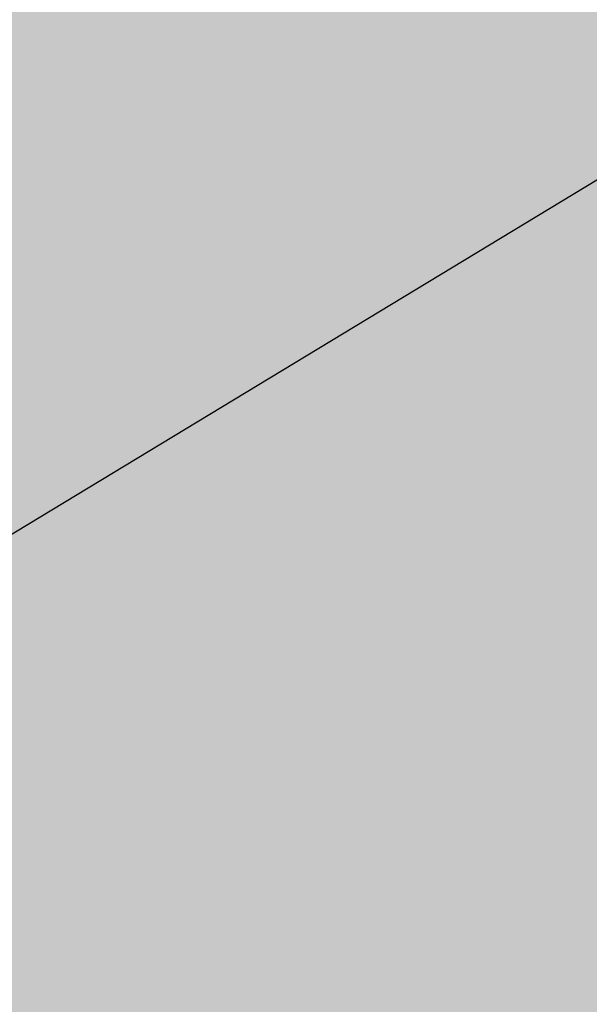
# Model space of a CAD drawing. Units: millimetres. Extents: x -22994 to 29398, y -19990 to 20176.
# Tile 62 of 135: x 223.108 to 225.272, y 83.328 to 87.071. Entities that reach past the tile are written whole.
import ezdxf
from ezdxf import colors
from ezdxf.entities.mleader import LeaderData, LeaderLine
from ezdxf.math import Vec2, Vec3

# ---------------------------------------------------------------- set-up
doc = ezdxf.new("R2010")
doc.units = ezdxf.units.MM
doc.header["$MEASUREMENT"] = 0
for name, color, linetype, lineweight in [('M-ANNO-TEXT', 7, 'Continuous', 25), ('M-DIMS', 2, 'Continuous', 18), ('M-EQPM', 7, 'Continuous', 25), ('M-EQPM-PATT', 7, 'Continuous', 18)]:
    doc.layers.add(name, color=color, linetype=linetype, lineweight=lineweight)
doc.styles.get("Standard").update_dxf_attribs({"font": 'arial.ttf'})
doc.dimstyles.get("Standard").update_dxf_attribs({"dimtxt": 0.18, "dimasz": 10000, "dimexe": 0.18, "dimexo": 0.0625, "dimgap": 0.09, "dimtad": 0, "dimtih": 1, "dimtoh": 1, "dimdec": 0, "dimzin": 0, "dimdsep": 46, "dimtxsty": 'Standard', "dimcen": 0.09, "dimadec": 0, "dimazin": 0, "dimtfac": 1, "dimtdec": 0, "dimtofl": 0, "dimtmove": 0, "dimatfit": 3, "dimfxl": 1, "dimtolj": 1, "dimtzin": 0, "dimlwd": 30, "dimarcsym": 0})

# ---------------------------------------------------------------- blocks, each defined once
blk = doc.blocks.new('*D2')
at = {"layer": 'Defpoints', "color": 0, "transparency": 16777216}
for p in [(6.6773, 10.2713), (290.852, 10.2713), (290.852, -5.0787)]:
    blk.add_point(p, dxfattribs=at)
at = {"layer": 'M-DIMS', "color": 0, "lineweight": -2, "transparency": 16777216}
for p, q in [((6.6773, 10.2088), (6.6773, -5.2587)), ((290.852, 10.2088), (290.852, -5.2587))]:
    blk.add_line(p, q, dxfattribs=at)
at = {"layer": 'M-DIMS', "color": 0, "lineweight": 30, "transparency": 16777216}
for p, q in [((-9993.3227, -5.0787), (-19993.3227, -5.0787)), ((10290.852, -5.0787), (20290.852, -5.0787))]:
    blk.add_line(p, q, dxfattribs=at)
at = {"layer": 'M-DIMS', "color": 0, "transparency": 16777216}
for points in [[(-9993.3227, 1661.5879), (-9993.3227, -1671.7454), (6.6773, -5.0787)], [(10290.852, 1661.5879), (10290.852, -1671.7454), (290.852, -5.0787)]]:
    blk.add_solid(points, dxfattribs=at)
at = {"layer": 'M-DIMS', "color": 0, "transparency": 16777216, "insert": (148.7647, -5.0787), "char_height": 0.18, "attachment_point": 5}
blk.add_mtext('\\A1;284.2', dxfattribs=at)
blk = doc.blocks.new('*D3')
at = {"layer": 'Defpoints', "color": 0, "transparency": 16777216}
for p in [(110.2647, 204.1654), (110.2647, 176.3662), (95.8327, 127.967)]:
    blk.add_point(p, dxfattribs=at)
at = {"layer": 'M-DIMS', "color": 0, "lineweight": -2, "transparency": 16777216}
for p, q in [((95.8327, 128.0295), (95.8327, 204.3454)), ((110.2647, 176.4287), (110.2647, 204.3454))]:
    blk.add_line(p, q, dxfattribs=at)
at = {"layer": 'M-DIMS', "color": 0, "lineweight": 30, "transparency": 16777216}
for p, q in [((-9904.1673, 204.1654), (-19904.1673, 204.1654)), ((10110.2647, 204.1654), (20110.2647, 204.1654))]:
    blk.add_line(p, q, dxfattribs=at)
at = {"layer": 'M-DIMS', "color": 0, "transparency": 16777216}
for points in [[(-9904.1673, 1870.8321), (-9904.1673, -1462.5013), (95.8327, 204.1654)], [(10110.2647, 1870.8321), (10110.2647, -1462.5013), (110.2647, 204.1654)]]:
    blk.add_solid(points, dxfattribs=at)
at = {"layer": 'M-DIMS', "color": 0, "transparency": 16777216, "insert": (103.0487, 204.1654), "char_height": 0.18, "attachment_point": 5}
blk.add_mtext('\\A1;14.432', dxfattribs=at)
blk = doc.blocks.new('*D4')
at = {"layer": 'Defpoints', "color": 0, "transparency": 16777216}
for p in [(116.2647, 204.1654), (110.2647, 176.3662), (116.2647, 176.3662)]:
    blk.add_point(p, dxfattribs=at)
at = {"layer": 'M-DIMS', "color": 0, "lineweight": -2, "transparency": 16777216}
for p, q in [((110.2647, 176.4287), (110.2647, 204.3454)), ((116.2647, 176.4287), (116.2647, 204.3454))]:
    blk.add_line(p, q, dxfattribs=at)
at = {"layer": 'M-DIMS', "color": 0, "lineweight": 30, "transparency": 16777216}
for p, q in [((-9889.7353, 204.1654), (-19889.7353, 204.1654)), ((10116.2647, 204.1654), (20116.2647, 204.1654))]:
    blk.add_line(p, q, dxfattribs=at)
at = {"layer": 'M-DIMS', "color": 0, "transparency": 16777216}
for points in [[(-9889.7353, 1870.8321), (-9889.7353, -1462.5013), (110.2647, 204.1654)], [(10116.2647, 1870.8321), (10116.2647, -1462.5013), (116.2647, 204.1654)]]:
    blk.add_solid(points, dxfattribs=at)
at = {"layer": 'M-DIMS', "color": 0, "transparency": 16777216, "insert": (113.2647, 204.1654), "char_height": 0.18, "attachment_point": 5}
blk.add_mtext('\\A1;6', dxfattribs=at)
blk = doc.blocks.new('*D5')
at = {"layer": 'Defpoints', "color": 0, "transparency": 16777216}
for p in [(181.2647, 204.1654), (116.2647, 176.3662), (181.2647, 176.3662)]:
    blk.add_point(p, dxfattribs=at)
at = {"layer": 'M-DIMS', "color": 0, "lineweight": -2, "transparency": 16777216}
for p, q in [((116.2647, 176.4287), (116.2647, 204.3454)), ((181.2647, 176.4287), (181.2647, 204.3454))]:
    blk.add_line(p, q, dxfattribs=at)
at = {"layer": 'M-DIMS', "color": 0, "lineweight": 30, "transparency": 16777216}
for p, q in [((-9883.7353, 204.1654), (-19883.7353, 204.1654)), ((10181.2647, 204.1654), (20181.2647, 204.1654))]:
    blk.add_line(p, q, dxfattribs=at)
at = {"layer": 'M-DIMS', "color": 0, "transparency": 16777216}
for points in [[(-9883.7353, 1870.8321), (-9883.7353, -1462.5013), (116.2647, 204.1654)], [(10181.2647, 1870.8321), (10181.2647, -1462.5013), (181.2647, 204.1654)]]:
    blk.add_solid(points, dxfattribs=at)
at = {"layer": 'M-DIMS', "color": 0, "transparency": 16777216, "insert": (148.7647, 204.1654), "char_height": 0.18, "attachment_point": 5}
blk.add_mtext('\\A1;65', dxfattribs=at)
blk = doc.blocks.new('*D6')
at = {"layer": 'Defpoints', "color": 0, "transparency": 16777216}
for p in [(187.2647, 204.1654), (181.2647, 176.3662), (187.2647, 176.3662)]:
    blk.add_point(p, dxfattribs=at)
at = {"layer": 'M-DIMS', "color": 0, "lineweight": -2, "transparency": 16777216}
for p, q in [((181.2647, 176.4287), (181.2647, 204.3454)), ((187.2647, 176.4287), (187.2647, 204.3454))]:
    blk.add_line(p, q, dxfattribs=at)
at = {"layer": 'M-DIMS', "color": 0, "lineweight": 30, "transparency": 16777216}
for p, q in [((-9818.7353, 204.1654), (-19818.7353, 204.1654)), ((10187.2647, 204.1654), (20187.2647, 204.1654))]:
    blk.add_line(p, q, dxfattribs=at)
at = {"layer": 'M-DIMS', "color": 0, "transparency": 16777216}
for points in [[(-9818.7353, 1870.8321), (-9818.7353, -1462.5013), (181.2647, 204.1654)], [(10187.2647, 1870.8321), (10187.2647, -1462.5013), (187.2647, 204.1654)]]:
    blk.add_solid(points, dxfattribs=at)
at = {"layer": 'M-DIMS', "color": 0, "transparency": 16777216, "insert": (184.2647, 204.1654), "char_height": 0.18, "attachment_point": 5}
blk.add_mtext('\\A1;6', dxfattribs=at)
blk = doc.blocks.new('*D7')
at = {"layer": 'Defpoints', "color": 0, "transparency": 16777216}
for p in [(201.6967, 204.1654), (187.2647, 176.3662), (201.6967, 127.967)]:
    blk.add_point(p, dxfattribs=at)
at = {"layer": 'M-DIMS', "color": 0, "lineweight": -2, "transparency": 16777216}
for p, q in [((187.2647, 176.4287), (187.2647, 204.3454)), ((201.6967, 128.0295), (201.6967, 204.3454))]:
    blk.add_line(p, q, dxfattribs=at)
at = {"layer": 'M-DIMS', "color": 0, "lineweight": 30, "transparency": 16777216}
for p, q in [((-9812.7353, 204.1654), (-19812.7353, 204.1654)), ((10201.6967, 204.1654), (20201.6967, 204.1654))]:
    blk.add_line(p, q, dxfattribs=at)
at = {"layer": 'M-DIMS', "color": 0, "transparency": 16777216}
for points in [[(-9812.7353, 1870.8321), (-9812.7353, -1462.5013), (187.2647, 204.1654)], [(10201.6967, 1870.8321), (10201.6967, -1462.5013), (201.6967, 204.1654)]]:
    blk.add_solid(points, dxfattribs=at)
at = {"layer": 'M-DIMS', "color": 0, "transparency": 16777216, "insert": (194.4807, 204.1654), "char_height": 0.18, "attachment_point": 5}
blk.add_mtext('\\A1;14.432', dxfattribs=at)
blk = doc.blocks.new('*D8')
at = {"layer": 'Defpoints', "color": 0, "transparency": 16777216}
for p in [(227.6485, 204.1654), (227.6485, 146.7296), (201.6967, 127.967)]:
    blk.add_point(p, dxfattribs=at)
at = {"layer": 'M-DIMS', "color": 0, "lineweight": -2, "transparency": 16777216}
for p, q in [((201.6967, 128.0295), (201.6967, 204.3454)), ((227.6485, 146.7921), (227.6485, 204.3454))]:
    blk.add_line(p, q, dxfattribs=at)
at = {"layer": 'M-DIMS', "color": 0, "lineweight": 30, "transparency": 16777216}
for p, q in [((-9798.3033, 204.1654), (-19798.3033, 204.1654)), ((10227.6485, 204.1654), (20227.6485, 204.1654))]:
    blk.add_line(p, q, dxfattribs=at)
at = {"layer": 'M-DIMS', "color": 0, "transparency": 16777216}
for points in [[(-9798.3033, 1870.8321), (-9798.3033, -1462.5013), (201.6967, 204.1654)], [(10227.6485, 1870.8321), (10227.6485, -1462.5013), (227.6485, 204.1654)]]:
    blk.add_solid(points, dxfattribs=at)
at = {"layer": 'M-DIMS', "color": 0, "transparency": 16777216, "insert": (214.6726, 204.1654), "char_height": 0.18, "attachment_point": 5}
blk.add_mtext('\\A1;25.95', dxfattribs=at)
blk = doc.blocks.new('*D9')
at = {"layer": 'Defpoints', "color": 0, "transparency": 16777216}
for p in [(187.2647, 176.3662), (306.202, 176.3662), (290.852, 10.2713)]:
    blk.add_point(p, dxfattribs=at)
at = {"layer": 'M-DIMS', "color": 0, "lineweight": 30, "transparency": 16777216}
for p, q in [((306.202, 10176.3662), (306.202, 20176.3662)), ((306.202, -9989.7287), (306.202, -19989.7287))]:
    blk.add_line(p, q, dxfattribs=at)
at = {"layer": 'M-DIMS', "color": 0, "lineweight": -2, "transparency": 16777216}
for p, q in [((187.3272, 176.3662), (306.382, 176.3662)), ((290.9145, 10.2713), (306.382, 10.2713))]:
    blk.add_line(p, q, dxfattribs=at)
at = {"layer": 'M-DIMS', "color": 0, "transparency": 16777216}
for points in [[(-1360.4646, 10176.3662), (1972.8687, 10176.3662), (306.202, 176.3662)], [(-1360.4646, -9989.7287), (1972.8687, -9989.7287), (306.202, 10.2713)]]:
    blk.add_solid(points, dxfattribs=at)
at = {"layer": 'M-DIMS', "color": 0, "transparency": 16777216, "insert": (306.202, 93.3187), "char_height": 0.18, "attachment_point": 5}
blk.add_mtext('\\A1;166.1', dxfattribs=at)
blk = doc.blocks.new('*D10')
at = {"layer": 'Defpoints', "color": 0, "transparency": 16777216}
for p in [(125.6498, 136.0713), (133.3459, 136.0713), (133.3459, -5.0787)]:
    blk.add_point(p, dxfattribs=at)
at = {"layer": 'M-DIMS', "color": 0, "lineweight": -2, "transparency": 16777216}
for p, q in [((125.6498, 136.0088), (125.6498, -5.2587)), ((133.3459, 136.0088), (133.3459, -5.2587))]:
    blk.add_line(p, q, dxfattribs=at)
at = {"layer": 'M-DIMS', "color": 0, "lineweight": 30, "transparency": 16777216}
for p, q in [((-9874.3502, -5.0787), (-19874.3502, -5.0787)), ((10133.3459, -5.0787), (20133.3459, -5.0787))]:
    blk.add_line(p, q, dxfattribs=at)
at = {"layer": 'M-DIMS', "color": 0, "transparency": 16777216}
for points in [[(-9874.3502, 1661.5879), (-9874.3502, -1671.7454), (125.6498, -5.0787)], [(10133.3459, 1661.5879), (10133.3459, -1671.7454), (133.3459, -5.0787)]]:
    blk.add_solid(points, dxfattribs=at)
at = {"layer": 'M-DIMS', "color": 0, "transparency": 16777216, "insert": (129.4978, -5.0787), "char_height": 0.18, "attachment_point": 5}
blk.add_mtext('\\A1;7.696', dxfattribs=at)
blk = doc.blocks.new('*D11')
at = {"layer": 'Defpoints', "color": 0, "transparency": 16777216}
for p in [(133.3459, 136.0713), (135.6498, 136.0713), (135.6498, -5.0787)]:
    blk.add_point(p, dxfattribs=at)
at = {"layer": 'M-DIMS', "color": 0, "lineweight": -2, "transparency": 16777216}
for p, q in [((133.3459, 136.0088), (133.3459, -5.2587)), ((135.6498, 136.0088), (135.6498, -5.2587))]:
    blk.add_line(p, q, dxfattribs=at)
at = {"layer": 'M-DIMS', "color": 0, "lineweight": 30, "transparency": 16777216}
for p, q in [((-9866.6541, -5.0787), (-19866.6541, -5.0787)), ((10135.6498, -5.0787), (20135.6498, -5.0787))]:
    blk.add_line(p, q, dxfattribs=at)
at = {"layer": 'M-DIMS', "color": 0, "transparency": 16777216}
for points in [[(-9866.6541, 1661.5879), (-9866.6541, -1671.7454), (133.3459, -5.0787)], [(10135.6498, 1661.5879), (10135.6498, -1671.7454), (135.6498, -5.0787)]]:
    blk.add_solid(points, dxfattribs=at)
at = {"layer": 'M-DIMS', "color": 0, "transparency": 16777216, "insert": (134.4978, -5.0787), "char_height": 0.18, "attachment_point": 5}
blk.add_mtext('\\A1;2.304', dxfattribs=at)
blk = doc.blocks.new('*D12')
at = {"layer": 'Defpoints', "color": 0, "transparency": 16777216}
for p in [(135.6498, 136.0713), (145.6498, 136.0713), (145.6498, -5.0787)]:
    blk.add_point(p, dxfattribs=at)
at = {"layer": 'M-DIMS', "color": 0, "lineweight": -2, "transparency": 16777216}
for p, q in [((135.6498, 136.0088), (135.6498, -5.2587)), ((145.6498, 136.0088), (145.6498, -5.2587))]:
    blk.add_line(p, q, dxfattribs=at)
at = {"layer": 'M-DIMS', "color": 0, "lineweight": 30, "transparency": 16777216}
for p, q in [((-9864.3502, -5.0787), (-19864.3502, -5.0787)), ((10145.6498, -5.0787), (20145.6498, -5.0787))]:
    blk.add_line(p, q, dxfattribs=at)
at = {"layer": 'M-DIMS', "color": 0, "transparency": 16777216}
for points in [[(-9864.3502, 1661.5879), (-9864.3502, -1671.7454), (135.6498, -5.0787)], [(10145.6498, 1661.5879), (10145.6498, -1671.7454), (145.6498, -5.0787)]]:
    blk.add_solid(points, dxfattribs=at)
at = {"layer": 'M-DIMS', "color": 0, "transparency": 16777216, "insert": (140.6498, -5.0787), "char_height": 0.18, "attachment_point": 5}
blk.add_mtext('\\A1;10', dxfattribs=at)
blk = doc.blocks.new('*D13')
at = {"layer": 'Defpoints', "color": 0, "transparency": 16777216}
for p in [(145.6498, 136.0713), (155.6498, 136.0713), (155.6498, -5.0787)]:
    blk.add_point(p, dxfattribs=at)
at = {"layer": 'M-DIMS', "color": 0, "lineweight": -2, "transparency": 16777216}
for p, q in [((145.6498, 136.0088), (145.6498, -5.2587)), ((155.6498, 136.0088), (155.6498, -5.2587))]:
    blk.add_line(p, q, dxfattribs=at)
at = {"layer": 'M-DIMS', "color": 0, "lineweight": 30, "transparency": 16777216}
for p, q in [((-9854.3502, -5.0787), (-19854.3502, -5.0787)), ((10155.6498, -5.0787), (20155.6498, -5.0787))]:
    blk.add_line(p, q, dxfattribs=at)
at = {"layer": 'M-DIMS', "color": 0, "transparency": 16777216}
for points in [[(-9854.3502, 1661.5879), (-9854.3502, -1671.7454), (145.6498, -5.0787)], [(10155.6498, 1661.5879), (10155.6498, -1671.7454), (155.6498, -5.0787)]]:
    blk.add_solid(points, dxfattribs=at)
at = {"layer": 'M-DIMS', "color": 0, "transparency": 16777216, "insert": (150.6498, -5.0787), "char_height": 0.18, "attachment_point": 5}
blk.add_mtext('\\A1;10', dxfattribs=at)
blk = doc.blocks.new('*D14')
at = {"layer": 'Defpoints', "color": 0, "transparency": 16777216}
for p in [(155.6498, 136.0713), (165.6498, 136.0713), (165.6498, -5.0787)]:
    blk.add_point(p, dxfattribs=at)
at = {"layer": 'M-DIMS', "color": 0, "lineweight": -2, "transparency": 16777216}
for p, q in [((155.6498, 136.0088), (155.6498, -5.2587)), ((165.6498, 136.0088), (165.6498, -5.2587))]:
    blk.add_line(p, q, dxfattribs=at)
at = {"layer": 'M-DIMS', "color": 0, "lineweight": 30, "transparency": 16777216}
for p, q in [((-9844.3502, -5.0787), (-19844.3502, -5.0787)), ((10165.6498, -5.0787), (20165.6498, -5.0787))]:
    blk.add_line(p, q, dxfattribs=at)
at = {"layer": 'M-DIMS', "color": 0, "transparency": 16777216}
for points in [[(-9844.3502, 1661.5879), (-9844.3502, -1671.7454), (155.6498, -5.0787)], [(10165.6498, 1661.5879), (10165.6498, -1671.7454), (165.6498, -5.0787)]]:
    blk.add_solid(points, dxfattribs=at)
at = {"layer": 'M-DIMS', "color": 0, "transparency": 16777216, "insert": (160.6498, -5.0787), "char_height": 0.18, "attachment_point": 5}
blk.add_mtext('\\A1;10', dxfattribs=at)
blk = doc.blocks.new('*D15')
at = {"layer": 'Defpoints', "color": 0, "transparency": 16777216}
for p in [(173.3459, 154.788), (173.3459, 136.0713), (306.202, 136.0713)]:
    blk.add_point(p, dxfattribs=at)
at = {"layer": 'M-DIMS', "color": 0, "lineweight": 30, "transparency": 16777216}
for p, q in [((306.202, 10154.788), (306.202, 20154.788)), ((306.202, -9863.9287), (306.202, -19863.9287))]:
    blk.add_line(p, q, dxfattribs=at)
at = {"layer": 'M-DIMS', "color": 0, "lineweight": -2, "transparency": 16777216}
for p, q in [((173.4084, 154.788), (306.382, 154.788)), ((173.4084, 136.0713), (306.382, 136.0713))]:
    blk.add_line(p, q, dxfattribs=at)
at = {"layer": 'M-DIMS', "color": 0, "transparency": 16777216}
for points in [[(-1360.4646, 10154.788), (1972.8687, 10154.788), (306.202, 154.788)], [(-1360.4646, -9863.9287), (1972.8687, -9863.9287), (306.202, 136.0713)]]:
    blk.add_solid(points, dxfattribs=at)
at = {"layer": 'M-DIMS', "color": 0, "transparency": 16777216, "insert": (306.202, 145.4297), "char_height": 0.18, "attachment_point": 5}
blk.add_mtext('\\A1;18.717', dxfattribs=at)
blk = doc.blocks.new('*D16')
at = {"layer": 'Defpoints', "color": 0, "transparency": 16777216}
for p in [(120.1702, 204.1654), (110.4658, 48.0349), (120.1702, 48.0349)]:
    blk.add_point(p, dxfattribs=at)
at = {"layer": 'M-DIMS', "color": 0, "lineweight": -2, "transparency": 16777216}
for p, q in [((110.4658, 48.0974), (110.4658, 204.3454)), ((120.1702, 48.0974), (120.1702, 204.3454))]:
    blk.add_line(p, q, dxfattribs=at)
at = {"layer": 'M-DIMS', "color": 0, "lineweight": 30, "transparency": 16777216}
for p, q in [((-9889.5342, 204.1654), (-19889.5342, 204.1654)), ((10120.1702, 204.1654), (20120.1702, 204.1654))]:
    blk.add_line(p, q, dxfattribs=at)
at = {"layer": 'M-DIMS', "color": 0, "transparency": 16777216}
for points in [[(-9889.5342, 1870.8321), (-9889.5342, -1462.5013), (110.4658, 204.1654)], [(10120.1702, 1870.8321), (10120.1702, -1462.5013), (120.1702, 204.1654)]]:
    blk.add_solid(points, dxfattribs=at)
at = {"layer": 'M-DIMS', "color": 0, "transparency": 16777216, "insert": (115.318, 204.1654), "char_height": 0.18, "attachment_point": 5}
blk.add_mtext('\\A1;9.704', dxfattribs=at)
blk = doc.blocks.new('*D17')
at = {"layer": 'Defpoints', "color": 0, "transparency": 16777216}
for p in [(126.1702, 204.1654), (120.1702, 48.0349), (126.1702, 48.0349)]:
    blk.add_point(p, dxfattribs=at)
at = {"layer": 'M-DIMS', "color": 0, "lineweight": -2, "transparency": 16777216}
for p, q in [((120.1702, 48.0974), (120.1702, 204.3454)), ((126.1702, 48.0974), (126.1702, 204.3454))]:
    blk.add_line(p, q, dxfattribs=at)
at = {"layer": 'M-DIMS', "color": 0, "lineweight": 30, "transparency": 16777216}
for p, q in [((-9879.8298, 204.1654), (-19879.8298, 204.1654)), ((10126.1702, 204.1654), (20126.1702, 204.1654))]:
    blk.add_line(p, q, dxfattribs=at)
at = {"layer": 'M-DIMS', "color": 0, "transparency": 16777216}
for points in [[(-9879.8298, 1870.8321), (-9879.8298, -1462.5013), (120.1702, 204.1654)], [(10126.1702, 1870.8321), (10126.1702, -1462.5013), (126.1702, 204.1654)]]:
    blk.add_solid(points, dxfattribs=at)
at = {"layer": 'M-DIMS', "color": 0, "transparency": 16777216, "insert": (123.1702, 204.1654), "char_height": 0.18, "attachment_point": 5}
blk.add_mtext('\\A1;6', dxfattribs=at)
blk = doc.blocks.new('*D18')
at = {"layer": 'Defpoints', "color": 0, "transparency": 16777216}
for p in [(132.1702, 204.1654), (126.1702, 48.0349), (132.1702, 48.0349)]:
    blk.add_point(p, dxfattribs=at)
at = {"layer": 'M-DIMS', "color": 0, "lineweight": -2, "transparency": 16777216}
for p, q in [((126.1702, 48.0974), (126.1702, 204.3454)), ((132.1702, 48.0974), (132.1702, 204.3454))]:
    blk.add_line(p, q, dxfattribs=at)
at = {"layer": 'M-DIMS', "color": 0, "lineweight": 30, "transparency": 16777216}
for p, q in [((-9873.8298, 204.1654), (-19873.8298, 204.1654)), ((10132.1702, 204.1654), (20132.1702, 204.1654))]:
    blk.add_line(p, q, dxfattribs=at)
at = {"layer": 'M-DIMS', "color": 0, "transparency": 16777216}
for points in [[(-9873.8298, 1870.8321), (-9873.8298, -1462.5013), (126.1702, 204.1654)], [(10132.1702, 1870.8321), (10132.1702, -1462.5013), (132.1702, 204.1654)]]:
    blk.add_solid(points, dxfattribs=at)
at = {"layer": 'M-DIMS', "color": 0, "transparency": 16777216, "insert": (129.1702, 204.1654), "char_height": 0.18, "attachment_point": 5}
blk.add_mtext('\\A1;6', dxfattribs=at)
blk = doc.blocks.new('*D19')
at = {"layer": 'Defpoints', "color": 0, "transparency": 16777216}
for p in [(138.1702, 204.1654), (132.1702, 48.0349), (138.1702, 48.0349)]:
    blk.add_point(p, dxfattribs=at)
at = {"layer": 'M-DIMS', "color": 0, "lineweight": -2, "transparency": 16777216}
for p, q in [((132.1702, 48.0974), (132.1702, 204.3454)), ((138.1702, 48.0974), (138.1702, 204.3454))]:
    blk.add_line(p, q, dxfattribs=at)
at = {"layer": 'M-DIMS', "color": 0, "lineweight": 30, "transparency": 16777216}
for p, q in [((-9867.8298, 204.1654), (-19867.8298, 204.1654)), ((10138.1702, 204.1654), (20138.1702, 204.1654))]:
    blk.add_line(p, q, dxfattribs=at)
at = {"layer": 'M-DIMS', "color": 0, "transparency": 16777216}
for points in [[(-9867.8298, 1870.8321), (-9867.8298, -1462.5013), (132.1702, 204.1654)], [(10138.1702, 1870.8321), (10138.1702, -1462.5013), (138.1702, 204.1654)]]:
    blk.add_solid(points, dxfattribs=at)
at = {"layer": 'M-DIMS', "color": 0, "transparency": 16777216, "insert": (135.1702, 204.1654), "char_height": 0.18, "attachment_point": 5}
blk.add_mtext('\\A1;6', dxfattribs=at)
blk = doc.blocks.new('*D20')
at = {"layer": 'Defpoints', "color": 0, "transparency": 16777216}
for p in [(144.1702, 204.1654), (138.1702, 48.0349), (144.1702, 48.0349)]:
    blk.add_point(p, dxfattribs=at)
at = {"layer": 'M-DIMS', "color": 0, "lineweight": -2, "transparency": 16777216}
for p, q in [((138.1702, 48.0974), (138.1702, 204.3454)), ((144.1702, 48.0974), (144.1702, 204.3454))]:
    blk.add_line(p, q, dxfattribs=at)
at = {"layer": 'M-DIMS', "color": 0, "lineweight": 30, "transparency": 16777216}
for p, q in [((-9861.8298, 204.1654), (-19861.8298, 204.1654)), ((10144.1702, 204.1654), (20144.1702, 204.1654))]:
    blk.add_line(p, q, dxfattribs=at)
at = {"layer": 'M-DIMS', "color": 0, "transparency": 16777216}
for points in [[(-9861.8298, 1870.8321), (-9861.8298, -1462.5013), (138.1702, 204.1654)], [(10144.1702, 1870.8321), (10144.1702, -1462.5013), (144.1702, 204.1654)]]:
    blk.add_solid(points, dxfattribs=at)
at = {"layer": 'M-DIMS', "color": 0, "transparency": 16777216, "insert": (141.1702, 204.1654), "char_height": 0.18, "attachment_point": 5}
blk.add_mtext('\\A1;6', dxfattribs=at)
blk = doc.blocks.new('*D21')
at = {"layer": 'Defpoints', "color": 0, "transparency": 16777216}
for p in [(149.1157, 204.1654), (144.1702, 48.0349), (149.1157, 48.0349)]:
    blk.add_point(p, dxfattribs=at)
at = {"layer": 'M-DIMS', "color": 0, "lineweight": -2, "transparency": 16777216}
for p, q in [((144.1702, 48.0974), (144.1702, 204.3454)), ((149.1157, 48.0974), (149.1157, 204.3454))]:
    blk.add_line(p, q, dxfattribs=at)
at = {"layer": 'M-DIMS', "color": 0, "lineweight": 30, "transparency": 16777216}
for p, q in [((-9855.8298, 204.1654), (-19855.8298, 204.1654)), ((10149.1157, 204.1654), (20149.1157, 204.1654))]:
    blk.add_line(p, q, dxfattribs=at)
at = {"layer": 'M-DIMS', "color": 0, "transparency": 16777216}
for points in [[(-9855.8298, 1870.8321), (-9855.8298, -1462.5013), (144.1702, 204.1654)], [(10149.1157, 1870.8321), (10149.1157, -1462.5013), (149.1157, 204.1654)]]:
    blk.add_solid(points, dxfattribs=at)
at = {"layer": 'M-DIMS', "color": 0, "transparency": 16777216, "insert": (146.6429, 204.1654), "char_height": 0.18, "attachment_point": 5}
blk.add_mtext('\\A1;4.945', dxfattribs=at)
blk = doc.blocks.new('*D22')
at = {"layer": 'Defpoints', "color": 0, "transparency": 16777216}
for p in [(149.1157, 30.9895), (155.1157, 30.9895), (155.1157, -5.0787)]:
    blk.add_point(p, dxfattribs=at)
at = {"layer": 'M-DIMS', "color": 0, "lineweight": -2, "transparency": 16777216}
for p, q in [((149.1157, 30.927), (149.1157, -5.2587)), ((155.1157, 30.927), (155.1157, -5.2587))]:
    blk.add_line(p, q, dxfattribs=at)
at = {"layer": 'M-DIMS', "color": 0, "lineweight": 30, "transparency": 16777216}
for p, q in [((-9850.8843, -5.0787), (-19850.8843, -5.0787)), ((10155.1157, -5.0787), (20155.1157, -5.0787))]:
    blk.add_line(p, q, dxfattribs=at)
at = {"layer": 'M-DIMS', "color": 0, "transparency": 16777216}
for points in [[(-9850.8843, 1661.5879), (-9850.8843, -1671.7454), (149.1157, -5.0787)], [(10155.1157, 1661.5879), (10155.1157, -1671.7454), (155.1157, -5.0787)]]:
    blk.add_solid(points, dxfattribs=at)
at = {"layer": 'M-DIMS', "color": 0, "transparency": 16777216, "insert": (152.1157, -5.0787), "char_height": 0.18, "attachment_point": 5}
blk.add_mtext('\\A1;6', dxfattribs=at)
blk = doc.blocks.new('*D23')
at = {"layer": 'Defpoints', "color": 0, "transparency": 16777216}
for p in [(155.1157, 30.9895), (161.1157, 30.9895), (161.1157, -5.0787)]:
    blk.add_point(p, dxfattribs=at)
at = {"layer": 'M-DIMS', "color": 0, "lineweight": -2, "transparency": 16777216}
for p, q in [((155.1157, 30.927), (155.1157, -5.2587)), ((161.1157, 30.927), (161.1157, -5.2587))]:
    blk.add_line(p, q, dxfattribs=at)
at = {"layer": 'M-DIMS', "color": 0, "lineweight": 30, "transparency": 16777216}
for p, q in [((-9844.8843, -5.0787), (-19844.8843, -5.0787)), ((10161.1157, -5.0787), (20161.1157, -5.0787))]:
    blk.add_line(p, q, dxfattribs=at)
at = {"layer": 'M-DIMS', "color": 0, "transparency": 16777216}
for points in [[(-9844.8843, 1661.5879), (-9844.8843, -1671.7454), (155.1157, -5.0787)], [(10161.1157, 1661.5879), (10161.1157, -1671.7454), (161.1157, -5.0787)]]:
    blk.add_solid(points, dxfattribs=at)
at = {"layer": 'M-DIMS', "color": 0, "transparency": 16777216, "insert": (158.1157, -5.0787), "char_height": 0.18, "attachment_point": 5}
blk.add_mtext('\\A1;6', dxfattribs=at)
blk = doc.blocks.new('*D24')
at = {"layer": 'Defpoints', "color": 0, "transparency": 16777216}
for p in [(161.1157, 30.9895), (166.4387, 30.9895), (166.4387, -5.0787)]:
    blk.add_point(p, dxfattribs=at)
at = {"layer": 'M-DIMS', "color": 0, "lineweight": -2, "transparency": 16777216}
for p, q in [((161.1157, 30.927), (161.1157, -5.2587)), ((166.4387, 30.927), (166.4387, -5.2587))]:
    blk.add_line(p, q, dxfattribs=at)
at = {"layer": 'M-DIMS', "color": 0, "lineweight": 30, "transparency": 16777216}
for p, q in [((-9838.8843, -5.0787), (-19838.8843, -5.0787)), ((10166.4387, -5.0787), (20166.4387, -5.0787))]:
    blk.add_line(p, q, dxfattribs=at)
at = {"layer": 'M-DIMS', "color": 0, "transparency": 16777216}
for points in [[(-9838.8843, 1661.5879), (-9838.8843, -1671.7454), (161.1157, -5.0787)], [(10166.4387, 1661.5879), (10166.4387, -1671.7454), (166.4387, -5.0787)]]:
    blk.add_solid(points, dxfattribs=at)
at = {"layer": 'M-DIMS', "color": 0, "transparency": 16777216, "insert": (163.7772, -5.0787), "char_height": 0.18, "attachment_point": 5}
blk.add_mtext('\\A1;5.323', dxfattribs=at)
blk = doc.blocks.new('*D25')
at = {"layer": 'Defpoints', "color": 0, "transparency": 16777216}
for p in [(166.4387, 30.9895), (172.4387, 30.9895), (172.4387, -5.0787)]:
    blk.add_point(p, dxfattribs=at)
at = {"layer": 'M-DIMS', "color": 0, "lineweight": -2, "transparency": 16777216}
for p, q in [((166.4387, 30.927), (166.4387, -5.2587)), ((172.4387, 30.927), (172.4387, -5.2587))]:
    blk.add_line(p, q, dxfattribs=at)
at = {"layer": 'M-DIMS', "color": 0, "lineweight": 30, "transparency": 16777216}
for p, q in [((-9833.5613, -5.0787), (-19833.5613, -5.0787)), ((10172.4387, -5.0787), (20172.4387, -5.0787))]:
    blk.add_line(p, q, dxfattribs=at)
at = {"layer": 'M-DIMS', "color": 0, "transparency": 16777216}
for points in [[(-9833.5613, 1661.5879), (-9833.5613, -1671.7454), (166.4387, -5.0787)], [(10172.4387, 1661.5879), (10172.4387, -1671.7454), (172.4387, -5.0787)]]:
    blk.add_solid(points, dxfattribs=at)
at = {"layer": 'M-DIMS', "color": 0, "transparency": 16777216, "insert": (169.4387, -5.0787), "char_height": 0.18, "attachment_point": 5}
blk.add_mtext('\\A1;6', dxfattribs=at)
blk = doc.blocks.new('*D26')
at = {"layer": 'Defpoints', "color": 0, "transparency": 16777216}
for p in [(172.4387, 30.9895), (178.4387, 30.9895), (178.4387, -5.0787)]:
    blk.add_point(p, dxfattribs=at)
at = {"layer": 'M-DIMS', "color": 0, "lineweight": -2, "transparency": 16777216}
for p, q in [((172.4387, 30.927), (172.4387, -5.2587)), ((178.4387, 30.927), (178.4387, -5.2587))]:
    blk.add_line(p, q, dxfattribs=at)
at = {"layer": 'M-DIMS', "color": 0, "lineweight": 30, "transparency": 16777216}
for p, q in [((-9827.5613, -5.0787), (-19827.5613, -5.0787)), ((10178.4387, -5.0787), (20178.4387, -5.0787))]:
    blk.add_line(p, q, dxfattribs=at)
at = {"layer": 'M-DIMS', "color": 0, "transparency": 16777216}
for points in [[(-9827.5613, 1661.5879), (-9827.5613, -1671.7454), (172.4387, -5.0787)], [(10178.4387, 1661.5879), (10178.4387, -1671.7454), (178.4387, -5.0787)]]:
    blk.add_solid(points, dxfattribs=at)
at = {"layer": 'M-DIMS', "color": 0, "transparency": 16777216, "insert": (175.4387, -5.0787), "char_height": 0.18, "attachment_point": 5}
blk.add_mtext('\\A1;6', dxfattribs=at)
blk = doc.blocks.new('*D27')
at = {"layer": 'Defpoints', "color": 0, "transparency": 16777216}
for p in [(178.4387, 30.9895), (188.1175, 30.9895), (188.1175, -5.0787)]:
    blk.add_point(p, dxfattribs=at)
at = {"layer": 'M-DIMS', "color": 0, "lineweight": -2, "transparency": 16777216}
for p, q in [((178.4387, 30.927), (178.4387, -5.2587)), ((188.1175, 30.927), (188.1175, -5.2587))]:
    blk.add_line(p, q, dxfattribs=at)
at = {"layer": 'M-DIMS', "color": 0, "lineweight": 30, "transparency": 16777216}
for p, q in [((-9821.5613, -5.0787), (-19821.5613, -5.0787)), ((10188.1175, -5.0787), (20188.1175, -5.0787))]:
    blk.add_line(p, q, dxfattribs=at)
at = {"layer": 'M-DIMS', "color": 0, "transparency": 16777216}
for points in [[(-9821.5613, 1661.5879), (-9821.5613, -1671.7454), (178.4387, -5.0787)], [(10188.1175, 1661.5879), (10188.1175, -1671.7454), (188.1175, -5.0787)]]:
    blk.add_solid(points, dxfattribs=at)
at = {"layer": 'M-DIMS', "color": 0, "transparency": 16777216, "insert": (183.2781, -5.0787), "char_height": 0.18, "attachment_point": 5}
blk.add_mtext('\\A1;9.679', dxfattribs=at)
blk = doc.blocks.new('*D28')
at = {"layer": 'Defpoints', "color": 0, "transparency": 16777216}
for p in [(188.1175, 48.0349), (306.202, 48.0349), (188.1175, 30.9895)]:
    blk.add_point(p, dxfattribs=at)
at = {"layer": 'M-DIMS', "color": 0, "lineweight": 30, "transparency": 16777216}
for p, q in [((306.202, 10048.0349), (306.202, 20048.0349)), ((306.202, -9969.0105), (306.202, -19969.0105))]:
    blk.add_line(p, q, dxfattribs=at)
at = {"layer": 'M-DIMS', "color": 0, "lineweight": -2, "transparency": 16777216}
for p, q in [((188.18, 48.0349), (306.382, 48.0349)), ((188.18, 30.9895), (306.382, 30.9895))]:
    blk.add_line(p, q, dxfattribs=at)
at = {"layer": 'M-DIMS', "color": 0, "transparency": 16777216}
for points in [[(-1360.4646, 10048.0349), (1972.8687, 10048.0349), (306.202, 48.0349)], [(-1360.4646, -9969.0105), (1972.8687, -9969.0105), (306.202, 30.9895)]]:
    blk.add_solid(points, dxfattribs=at)
at = {"layer": 'M-DIMS', "color": 0, "transparency": 16777216, "insert": (306.202, 39.5122), "char_height": 0.18, "attachment_point": 5}
blk.add_mtext('\\A1;17.045', dxfattribs=at)
blk = doc.blocks.new('*D29')
at = {"layer": 'Defpoints', "color": 0, "transparency": 16777216}
for p in [(36.8006, 80.045), (64.0296, 80.045)]:
    blk.add_point(p, dxfattribs=at)
at = {"layer": 'M-DIMS', "color": 0, "lineweight": -2, "transparency": 16777216}
for p, q in [((50.4151, 79.955), (50.4151, 80.135)), ((50.3251, 80.045), (50.5051, 80.045))]:
    blk.add_line(p, q, dxfattribs=at)
at = {"layer": 'M-DIMS', "color": 0, "lineweight": 30, "transparency": 16777216}
blk.add_line((20064.0296, 80.0303), (10064.0296, 80.0377), dxfattribs=at)
at = {"layer": 'M-DIMS', "color": 0, "transparency": 16777216}
blk.add_solid([(10064.0309, 1746.7043), (10064.0284, -1586.629), (64.0296, 80.045)], dxfattribs=at)
at = {"layer": 'M-DIMS', "color": 0, "transparency": 16777216, "insert": (20064.5213, 80.0303), "char_height": 0.18, "attachment_point": 5}
blk.add_mtext('\\A1;∅27.23', dxfattribs=at)
blk = doc.blocks.new('*D30')
at = {"layer": 'Defpoints', "color": 0, "transparency": 16777216}
for p in [(216.3148, 146.7291), (238.9821, 146.73)]:
    blk.add_point(p, dxfattribs=at)
at = {"layer": 'M-DIMS', "color": 0, "lineweight": 30, "transparency": 16777216}
blk.add_line((20238.9821, 147.4959), (10238.9821, 147.1129), dxfattribs=at)
at = {"layer": 'M-DIMS', "color": 0, "lineweight": -2, "transparency": 16777216}
for p, q in [((227.6485, 146.6396), (227.6485, 146.8196)), ((227.5585, 146.7296), (227.7385, 146.7296))]:
    blk.add_line(p, q, dxfattribs=at)
at = {"layer": 'M-DIMS', "color": 0, "transparency": 16777216}
blk.add_solid([(10238.9183, 1813.7796), (10239.0459, -1519.5537), (238.9821, 146.73)], dxfattribs=at)
at = {"layer": 'M-DIMS', "color": 0, "transparency": 16777216, "insert": (20239.5436, 147.4959), "char_height": 0.18, "attachment_point": 5}
blk.add_mtext('\\A1;∅22.667', dxfattribs=at)
blk = doc.blocks.new('*D31')
at = {"layer": 'Defpoints', "color": 0, "transparency": 16777216}
for p in [(223.1641, 146.7291), (232.1328, 146.73)]:
    blk.add_point(p, dxfattribs=at)
at = {"layer": 'M-DIMS', "color": 0, "lineweight": 30, "transparency": 16777216}
blk.add_line((20232.1327, 148.6656), (10232.1328, 147.6978), dxfattribs=at)
at = {"layer": 'M-DIMS', "color": 0, "lineweight": -2, "transparency": 16777216}
for p, q in [((227.6485, 146.6396), (227.6485, 146.8196)), ((227.5585, 146.7296), (227.7385, 146.7296))]:
    blk.add_line(p, q, dxfattribs=at)
at = {"layer": 'M-DIMS', "color": 0, "transparency": 16777216}
blk.add_solid([(10231.9715, 1814.3645), (10232.2941, -1518.9688), (232.1328, 146.73)], dxfattribs=at)
at = {"layer": 'M-DIMS', "color": 0, "transparency": 16777216, "insert": (20232.6245, 148.6656), "char_height": 0.18, "attachment_point": 5}
blk.add_mtext('\\A1;∅8.969', dxfattribs=at)
blk = doc.blocks.new('*D36')
at = {"layer": 'Defpoints', "color": 0, "transparency": 16777216}
for p in [(46.39, 31.3035), (46.3875, 26.5934)]:
    blk.add_point(p, dxfattribs=at)
at = {"layer": 'M-DIMS', "color": 0, "lineweight": 30, "transparency": 16777216}
for p, q in [((57.1499, 20031.3006), (51.77, 10031.302)), ((10057.1499, 20031.3006), (57.1499, 20031.3006))]:
    blk.add_line(p, q, dxfattribs=at)
at = {"layer": 'M-DIMS', "color": 0, "lineweight": -2, "transparency": 16777216}
for p, q in [((46.3887, 28.8585), (46.3887, 29.0385)), ((46.2987, 28.9485), (46.4787, 28.9485))]:
    blk.add_line(p, q, dxfattribs=at)
at = {"layer": 'M-DIMS', "color": 0, "transparency": 16777216}
blk.add_solid([(-1614.8965, 10032.1987), (1718.4364, 10030.4054), (46.39, 31.3035)], dxfattribs=at)
at = {"layer": 'M-DIMS', "color": 0, "transparency": 16777216, "insert": (10057.5542, 20031.3006), "char_height": 0.18, "attachment_point": 5}
blk.add_mtext('\\A1;∅4.71', dxfattribs=at)

msp = doc.modelspace()

# ---------------------------------------------------------------- hatches: boundary and pattern name
at = {"layer": 'M-EQPM-PATT'}
h = msp.add_hatch(color=256, dxfattribs=at)
h.set_gradient(color1=(205, 32, 39), color2=(205, 32, 39), tint=1)
h.paths.add_polyline_path([(116.2647, 150.3662), (116.2647, 170.3662), (116.2647, 176.3662), (110.2647, 176.3662), (110.2647, 152.0276), (95.8327, 127.967), (95.8327, 16.6063), (201.6967, 16.6063), (201.6967, 127.967), (187.2647, 152.0276), (187.2647, 176.3662), (181.2647, 176.3662), (181.2647, 170.3662), (181.2647, 150.3662), (195.6967, 126.3055), (195.6967, 22.6063), (101.8327, 22.6063), (101.8327, 126.3055)])
h.paths.add_polyline_path([(185.2208, 88.6347), (101.8327, 88.6347), (101.8327, 87.6347), (182.8066, 87.6347), (178.7313, 83.5594), (195.6967, 83.5594), (195.6967, 84.5594), (181.1455, 84.5594)], flags=17)
h.paths.add_polyline_path([(95.8327, 88.6347), (60.9779, 88.6347, -0.022855), (61.7178, 87.6347), (95.8327, 87.6347)])
h.paths.add_polyline_path([(215.6212, 86.5189), (215.6212, 80.5999), (220.5095, 83.5594)])
h.paths.add_polyline_path([(215.6212, 84.5594), (201.6967, 84.5594), (201.6967, 83.5594), (215.6212, 83.5594)])
h.paths.add_polyline_path([(225.3978, 86.5189), (220.5095, 83.5594), (225.3978, 80.5999)])
h.paths.add_polyline_path([(231.6256, 84.5594), (225.3978, 84.5594), (225.3978, 83.5594), (231.6256, 83.5594)])

# ---------------------------------------------------------------- linework, layer by layer
at = {"layer": 'M-EQPM'}
msp.add_lwpolyline([(225.3978, 86.5189), (215.6212, 80.5999), (215.6212, 86.5189), (225.3978, 80.5999)], close=True, dxfattribs=at)

# ---------------------------------------------------------------- dimensions: what is measured, and where the dimension line sits
at = {"layer": 'M-DIMS'}
for base, p1, p2, override, picture, middle in [((306.202, 176.3662), (290.852, 10.2713), (187.2647, 176.3662), {"dimdec": 1, "dimlfac": 1, "dimrnd": 0, "dimzin": 0, "dimdsep": 46, "dimlunit": 2}, '*D9', (306.202, 93.3187)), ((306.202, 136.0713), (173.3459, 154.788), (173.3459, 136.0713), {"dimdec": 3, "dimlfac": 1, "dimrnd": 0, "dimzin": 0, "dimdsep": 46, "dimlunit": 2}, '*D15', (306.202, 145.4297)), ((306.202, 48.0349), (188.1175, 30.9895), (188.1175, 48.0349), {"dimdec": 3, "dimlfac": 1, "dimrnd": 0, "dimzin": 0, "dimdsep": 46, "dimlunit": 2}, '*D28', (306.202, 39.5122))]:
    dim = msp.add_linear_dim(base=base, p1=p1, p2=p2, angle=90, dimstyle='Standard', override=override, dxfattribs=at)
    dim.commit()
    dim.dimension.update_dxf_attribs({"geometry": picture, "text_midpoint": middle})
for p1, p2, override, picture, middle in [((46.3875, 26.5934), (46.39, 31.3035), {"dimdec": 2, "dimlfac": 1, "dimrnd": 0, "dimzin": 0, "dimdsep": 46, "dimlunit": 2}, '*D36', (10057.5542, 20031.3006)), ((223.1641, 146.7291), (232.1328, 146.73), {"dimdec": 3, "dimlfac": 1, "dimrnd": 0, "dimzin": 0, "dimdsep": 46, "dimlunit": 2}, '*D31', (20232.1327, 148.6656)), ((216.3148, 146.7291), (238.9821, 146.73), {"dimdec": 3, "dimlfac": 1, "dimrnd": 0, "dimzin": 0, "dimdsep": 46, "dimlunit": 2}, '*D30', (20238.9821, 147.4959))]:
    dim = msp.add_diameter_dim_2p(p1=p1, p2=p2, dimstyle='Standard', override=override, dxfattribs=at)
    dim.commit()
    dim.dimension.update_dxf_attribs({"geometry": picture, "text_midpoint": middle, "dimtype": 163})
for base, p1, p2, override, picture, middle in [((110.2647, 204.1654), (95.8327, 127.967), (110.2647, 176.3662), {"dimdec": 3, "dimlfac": 1, "dimrnd": 0, "dimzin": 0, "dimdsep": 46, "dimlunit": 2}, '*D3', (103.0487, 204.1654)), ((116.2647, 204.1654), (110.2647, 176.3662), (116.2647, 176.3662), {"dimdec": 0, "dimlfac": 1, "dimrnd": 0, "dimzin": 0, "dimdsep": 46, "dimlunit": 2}, '*D4', (113.2647, 204.1654)), ((120.1702, 204.1654), (110.4658, 48.0349), (120.1702, 48.0349), {"dimdec": 3, "dimlfac": 1, "dimrnd": 0, "dimzin": 0, "dimdsep": 46, "dimlunit": 2}, '*D16', (115.318, 204.1654)), ((181.2647, 204.1654), (116.2647, 176.3662), (181.2647, 176.3662), {"dimdec": 0, "dimlfac": 1, "dimrnd": 0, "dimzin": 0, "dimdsep": 46, "dimlunit": 2}, '*D5', (148.7647, 204.1654)), ((126.1702, 204.1654), (120.1702, 48.0349), (126.1702, 48.0349), {"dimdec": 0, "dimlfac": 1, "dimrnd": 0, "dimzin": 0, "dimdsep": 46, "dimlunit": 2}, '*D17', (123.1702, 204.1654)), ((132.1702, 204.1654), (126.1702, 48.0349), (132.1702, 48.0349), {"dimdec": 0, "dimlfac": 1, "dimrnd": 0, "dimzin": 0, "dimdsep": 46, "dimlunit": 2}, '*D18', (129.1702, 204.1654)), ((138.1702, 204.1654), (132.1702, 48.0349), (138.1702, 48.0349), {"dimdec": 0, "dimlfac": 1, "dimrnd": 0, "dimzin": 0, "dimdsep": 46, "dimlunit": 2}, '*D19', (135.1702, 204.1654)), ((144.1702, 204.1654), (138.1702, 48.0349), (144.1702, 48.0349), {"dimdec": 0, "dimlfac": 1, "dimrnd": 0, "dimzin": 0, "dimdsep": 46, "dimlunit": 2}, '*D20', (141.1702, 204.1654)), ((149.11567, 204.16539), (144.17023, 48.03494), (149.11567, 48.03494), {"dimdec": 3, "dimlfac": 1, "dimrnd": 0, "dimzin": 0, "dimdsep": 46, "dimlunit": 2}, '*D21', (146.64295, 204.16539)), ((187.2647, 204.1654), (181.2647, 176.3662), (187.2647, 176.3662), {"dimdec": 0, "dimlfac": 1, "dimrnd": 0, "dimzin": 0, "dimdsep": 46, "dimlunit": 2}, '*D6', (184.2647, 204.1654)), ((201.6967, 204.1654), (187.2647, 176.3662), (201.6967, 127.967), {"dimdec": 3, "dimlfac": 1, "dimrnd": 0, "dimzin": 0, "dimdsep": 46, "dimlunit": 2}, '*D7', (194.4807, 204.1654)), ((227.6485, 204.1654), (201.6967, 127.967), (227.6485, 146.7296), {"dimdec": 2, "dimlfac": 1, "dimrnd": 0, "dimzin": 0, "dimdsep": 46, "dimlunit": 2}, '*D8', (214.6726, 204.1654)), ((290.852, -5.0787), (6.6773, 10.2713), (290.852, 10.2713), {"dimdec": 1, "dimlfac": 1, "dimrnd": 0, "dimzin": 0, "dimdsep": 46, "dimlunit": 2}, '*D2', (148.7647, -5.0787)), ((133.3459, -5.0787), (125.6498, 136.0713), (133.3459, 136.0713), {"dimdec": 3, "dimlfac": 1, "dimrnd": 0, "dimzin": 0, "dimdsep": 46, "dimlunit": 2}, '*D10', (129.4978, -5.0787)), ((135.6498, -5.0787), (133.3459, 136.0713), (135.6498, 136.0713), {"dimdec": 3, "dimlfac": 1, "dimrnd": 0, "dimzin": 0, "dimdsep": 46, "dimlunit": 2}, '*D11', (134.4978, -5.0787)), ((145.6498, -5.0787), (135.6498, 136.0713), (145.6498, 136.0713), {"dimdec": 0, "dimlfac": 1, "dimrnd": 0, "dimzin": 0, "dimdsep": 46, "dimlunit": 2}, '*D12', (140.6498, -5.0787)), ((155.6498, -5.0787), (145.6498, 136.0713), (155.6498, 136.0713), {"dimdec": 0, "dimlfac": 1, "dimrnd": 0, "dimzin": 0, "dimdsep": 46, "dimlunit": 2}, '*D13', (150.6498, -5.0787)), ((155.1157, -5.0787), (149.1157, 30.9895), (155.1157, 30.9895), {"dimdec": 0, "dimlfac": 1, "dimrnd": 0, "dimzin": 0, "dimdsep": 46, "dimlunit": 2}, '*D22', (152.1157, -5.0787)), ((161.1157, -5.0787), (155.1157, 30.9895), (161.1157, 30.9895), {"dimdec": 0, "dimlfac": 1, "dimrnd": 0, "dimzin": 0, "dimdsep": 46, "dimlunit": 2}, '*D23', (158.1157, -5.0787)), ((165.6498, -5.0787), (155.6498, 136.0713), (165.6498, 136.0713), {"dimdec": 0, "dimlfac": 1, "dimrnd": 0, "dimzin": 0, "dimdsep": 46, "dimlunit": 2}, '*D14', (160.6498, -5.0787)), ((166.4387, -5.0787), (161.1157, 30.9895), (166.4387, 30.9895), {"dimdec": 3, "dimlfac": 1, "dimrnd": 0, "dimzin": 0, "dimdsep": 46, "dimlunit": 2}, '*D24', (163.7772, -5.0787)), ((172.4387, -5.0787), (166.4387, 30.9895), (172.4387, 30.9895), {"dimdec": 0, "dimlfac": 1, "dimrnd": 0, "dimzin": 0, "dimdsep": 46, "dimlunit": 2}, '*D25', (169.4387, -5.0787)), ((178.4387, -5.0787), (172.4387, 30.9895), (178.4387, 30.9895), {"dimdec": 0, "dimlfac": 1, "dimrnd": 0, "dimzin": 0, "dimdsep": 46, "dimlunit": 2}, '*D26', (175.4387, -5.0787)), ((188.1175, -5.0787), (178.4387, 30.9895), (188.1175, 30.9895), {"dimdec": 3, "dimlfac": 1, "dimrnd": 0, "dimzin": 0, "dimdsep": 46, "dimlunit": 2}, '*D27', (183.2781, -5.0787))]:
    dim = msp.add_linear_dim(base=base, p1=p1, p2=p2, dimstyle='Standard', override=override, dxfattribs=at)
    dim.commit()
    dim.dimension.update_dxf_attribs({"geometry": picture, "text_midpoint": middle})
dim = msp.add_diameter_dim_2p(p1=(36.8006, 80.045), p2=(64.0296, 80.045), dimstyle='Standard', override={"dimdec": 2, "dimlfac": 1, "dimrnd": 0, "dimzin": 0, "dimdsep": 46, "dimlunit": 2}, dxfattribs=at)
dim.commit()
dim.dimension.update_dxf_attribs({"geometry": '*D29', "text_midpoint": (20064.0296, 80.0303)})

# ---------------------------------------------------------------- leaders
at = {"layer": 'M-ANNO-TEXT'}
ml = msp.add_multileader_mtext('Standard', dxfattribs=at)
ml.set_content('combustion chamber', color=256)
ml.set_leader_properties()
ml.build(insert=Vec2(0, 0))
ml.multileader.update_dxf_attribs({"dogleg_length": 0.36, "arrow_head_size": 200})
ctx = ml.context
ctx.base_point, ctx.char_height, ctx.arrow_head_size, ctx.landing_gap_size, ctx.plane_origin = Vec3(215.7321, 57.9149), 3, 200, 0.09, Vec3(189.1175, 57.9149)
notes = []
notes.append((ctx, [(0, (1, 1, 0), (215.3721, 57.9149), (1, 0), 0.36, [(0, [(189.1175, 57.9149)], 0, [])])]))
ctx.mtext.insert, ctx.mtext.flow_direction = Vec3(215.8221, 59.4394), 5
for ctx, leaders in notes:
    for number, flags, end, landing, length, lines in leaders:
        leader = LeaderData()
        leader.index, (leader.has_last_leader_line, leader.has_dogleg_vector, leader.attachment_direction) = number, flags
        leader.last_leader_point, leader.dogleg_vector, leader.dogleg_length = Vec3(end), Vec3(landing), length
        for number, points, colour, breaks in lines:
            line = LeaderLine()
            line.index, line.vertices, line.color, line.breaks = number, Vec3.list(points), colors.encode_raw_color(colour), breaks
            leader.lines.append(line)
        ctx.leaders.append(leader)

doc.saveas('drawing.dxf')
